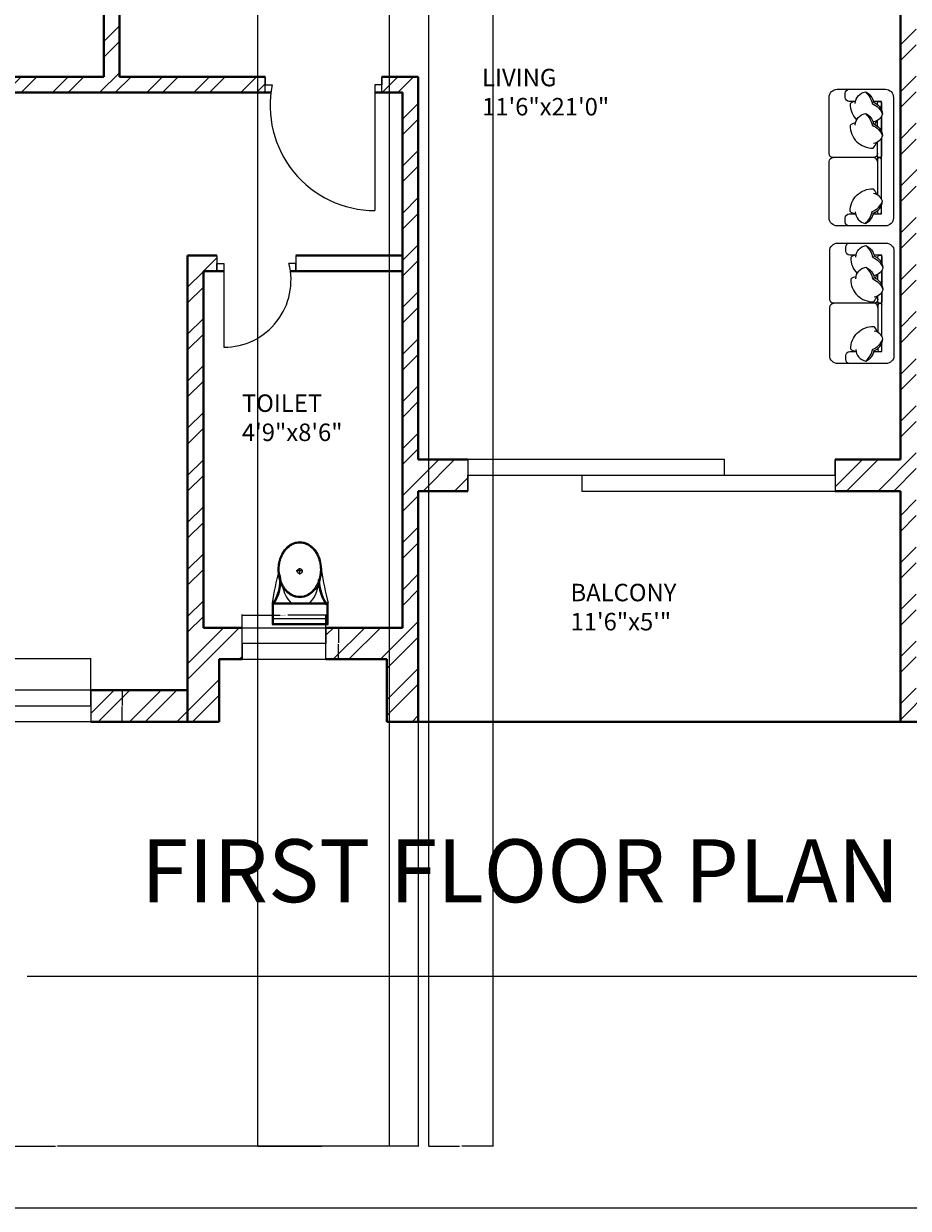
# Model space of a CAD drawing. Units: inches. Extents: x 1601 to 2297, y 1496 to 2631.
# Tile 4 of 57: x 1780 to 2033, y 1496 to 1835. Entities that reach past the tile are written whole.
import ezdxf

# ---------------------------------------------------------------- set-up
doc = ezdxf.new("R2010")
doc.units = ezdxf.units.IN
for name, color, linetype, lineweight in [('A-ANNO-DIMS', 2, 'Continuous', 18), ('A-ANNO-TTLB', 7, 'Continuous', 25), ('A-AREA-IDEN', 7, 'Continuous', 18), ('A-DOOR', 21, 'Continuous', 25), ('A-FLOR-FIXT', 9, 'Continuous', 20), ('A-FURN', 8, 'Continuous', 18), ('A-GLAZ', 161, 'Continuous', 20), ('A-WALL', 7, 'Continuous', 40), ('A-WALL-PATT', 215, 'Continuous', 13)]:
    doc.layers.add(name, color=color, linetype=linetype, lineweight=lineweight)
doc.styles.get("Standard").update_dxf_attribs({"font": 'arial.ttf'})
doc.dimstyles.get("Standard").update_dxf_attribs({"dimtxt": 0.18, "dimasz": 0.18, "dimexe": 0.18, "dimexo": 0.0625, "dimgap": 0.09, "dimtad": 0, "dimtih": 1, "dimtoh": 1, "dimdec": 4, "dimzin": 0, "dimdsep": 46, "dimtxsty": 'Standard', "dimcen": 0.09, "dimadec": 0, "dimazin": 0, "dimtfac": 1, "dimtdec": 4, "dimtofl": 0, "dimtmove": 0, "dimatfit": 3, "dimfxl": 1, "dimtolj": 1, "dimtzin": 0, "dimarcsym": 0})

# ---------------------------------------------------------------- blocks, each defined once
blk = doc.blocks.new('A$C31115884')
for p, q in [((283, 498), (223, 498)), ((258, 466), (258, 523)), ((0, 200), (0, 0)), ((520, 200), (0, 200)), ((10, 190), (10, 10)), ((510, 190), (10, 190)), ((510, 10), (510, 190)), ((520, 0), (520, 200)), ((510, 54), (0, 54)), ((10, 10), (510, 10)), ((0, 0), (520, 0))]:
    blk.add_line(p, q)
blk.add_circle((256, 496), 23.6)
for centre, radius, start, end in [((2778, -205), 2807, 165.4549, 171.7133), ((-295, 403), 365, 324.2091, 9.3499), ((-295, 403), 375, 324.2091, 9.3499), ((806, 403), 365, 170.6501, 215.7909), ((3237, 905), 2807, 188.2867, 194.5451), ((384, 406), 293, 190.2774, 224.1564), ((139, 406), 293, 315.8436, 2.6563), ((806, 403), 375, 179.2036, 215.7909)]:
    blk.add_arc(centre, radius, start, end)
blk.add_ellipse((256, 510), major_axis=(0, -261), ratio=0.772727)
blk.add_open_spline([(256, 259), (263, 259), (270, 260), (288, 262), (299, 265), (320, 273), (330, 278), (350, 291), (360, 299), (378, 316), (386, 326), (402, 347), (409, 358), (421, 383), (427, 395), (436, 422), (440, 436), (445, 465), (447, 480), (448, 509), (448, 524), (445, 553), (443, 568), (436, 596), (432, 610), (422, 636), (416, 649), (402, 672), (395, 683), (379, 703), (370, 712), (351, 728), (341, 735), (321, 746), (310, 751), (289, 757), (278, 759), (256, 761), (245, 761), (223, 757), (212, 754), (191, 746), (181, 741), (161, 728), (151, 720), (133, 703), (125, 693), (110, 672), (103, 660), (90, 636), (85, 623), (76, 596), (72, 582), (67, 553), (66, 538), (64, 509), (65, 494), (68, 465), (70, 450), (77, 422), (81, 408), (91, 382), (97, 370), (111, 346), (118, 335), (135, 316), (144, 307), (162, 291), (172, 284), (193, 273), (203, 269), (225, 262), (236, 260), (250, 259), (253, 259), (256, 259)], degree=3, knots=[0, 0, 0, 0, 0.110105, 0.110105, 0.285049, 0.285049, 0.459994, 0.459994, 0.634938, 0.634938, 0.809882, 0.809882, 0.984827, 0.984827, 1.159771, 1.159771, 1.334715, 1.334715, 1.50966, 1.50966, 1.684604, 1.684604, 1.859549, 1.859549, 2.034493, 2.034493, 2.209437, 2.209437, 2.384382, 2.384382, 2.559326, 2.559326, 2.73427, 2.73427, 2.909215, 2.909215, 3.084159, 3.084159, 3.259103, 3.259103, 3.434048, 3.434048, 3.608992, 3.608992, 3.783936, 3.783936, 3.958881, 3.958881, 4.133825, 4.133825, 4.30877, 4.30877, 4.483714, 4.483714, 4.658658, 4.658658, 4.833603, 4.833603, 5.008547, 5.008547, 5.183491, 5.183491, 5.358436, 5.358436, 5.53338, 5.53338, 5.708324, 5.708324, 5.883269, 5.883269, 6.058213, 6.058213, 6.233158, 6.233158, 6.283185, 6.283185, 6.283185, 6.283185])
blk = doc.blocks.new('WIN-60IN-JAMB9')
for p, q in [((4.5, 60), (0, 60)), ((0, 60), (9, 60)), ((0, 60), (0, 0)), ((4.5, 0), (4.5, 60)), ((9, 60), (9, 0)), ((0, 0), (9, 0)), ((9, 0), (4.5, 0))]:
    blk.add_line(p, q)
blk = doc.blocks.new('WIN-24IN-JAMB9')
for p, q in [((4.5, 24), (0, 24)), ((0, 24), (9, 24)), ((0, 24), (0, 0)), ((4.5, 0), (4.5, 24)), ((9, 24), (9, 0)), ((0, 0), (9, 0)), ((9, 0), (4.5, 0))]:
    blk.add_line(p, q)
blk = doc.blocks.new('*D14')
at = {"layer": 'A-ANNO-DIMS', "color": 0, "lineweight": -2, "transparency": 16777216}
for p, q in [((1739.33, 1644.39), (1739.33, 1653.51)), ((1739.51, 1653.33), (1768.22, 1653.33)), ((1799.15, 1653.33), (1770.45, 1653.33)), ((1799.33, 1644.39), (1799.33, 1653.51))]:
    blk.add_line(p, q, dxfattribs=at)
at = {"layer": 'A-ANNO-DIMS', "color": 0, "transparency": 16777216}
for points in [[(1739.51, 1653.36), (1739.51, 1653.3), (1739.33, 1653.33)], [(1799.15, 1653.36), (1799.15, 1653.3), (1799.33, 1653.33)]]:
    blk.add_solid(points, dxfattribs=at)
at = {"layer": 'Defpoints', "color": 0, "transparency": 16777216}
for p in [(1799.33, 1653.33), (1739.33, 1644.33), (1799.33, 1644.33)]:
    blk.add_point(p, dxfattribs=at)
at = {"layer": 'A-ANNO-DIMS', "color": 0, "transparency": 16777216, "insert": (1769.33, 1653.33), "char_height": 0.18, "attachment_point": 5}
blk.add_mtext('\\A1;WINDOW 60 TYP.', dxfattribs=at)
blk = doc.blocks.new('*D15')
at = {"layer": 'A-ANNO-DIMS', "color": 0, "lineweight": -2, "transparency": 16777216}
for p, q in [((1799.4, 1644.33), (1808.51, 1644.33)), ((1808.33, 1644.15), (1808.33, 1640.01)), ((1808.33, 1635.51), (1808.33, 1639.64)), ((1799.4, 1635.33), (1808.51, 1635.33))]:
    blk.add_line(p, q, dxfattribs=at)
at = {"layer": 'A-ANNO-DIMS', "color": 0, "transparency": 16777216}
for points in [[(1808.3, 1644.15), (1808.36, 1644.15), (1808.33, 1644.33)], [(1808.3, 1635.51), (1808.36, 1635.51), (1808.33, 1635.33)]]:
    blk.add_solid(points, dxfattribs=at)
at = {"layer": 'Defpoints', "color": 0, "transparency": 16777216}
for p in [(1799.33, 1644.33), (1799.33, 1635.33), (1808.33, 1635.33)]:
    blk.add_point(p, dxfattribs=at)
at = {"layer": 'A-ANNO-DIMS', "color": 0, "transparency": 16777216, "insert": (1808.33, 1639.83), "char_height": 0.18, "attachment_point": 5}
blk.add_mtext('\\A1;9 TYP.', dxfattribs=at)
blk = doc.blocks.new('*D26')
at = {"layer": 'A-ANNO-DIMS', "color": 0, "lineweight": -2, "transparency": 16777216}
for p, q in [((1842.62, 1662.27), (1842.62, 1665.98)), ((1842.8, 1665.8), (1853.5, 1665.8)), ((1866.44, 1665.8), (1855.74, 1665.8)), ((1866.62, 1662.27), (1866.62, 1665.98))]:
    blk.add_line(p, q, dxfattribs=at)
at = {"layer": 'A-ANNO-DIMS', "color": 0, "transparency": 16777216}
for points in [[(1842.8, 1665.83), (1842.8, 1665.77), (1842.62, 1665.8)], [(1866.44, 1665.83), (1866.44, 1665.77), (1866.62, 1665.8)]]:
    blk.add_solid(points, dxfattribs=at)
at = {"layer": 'Defpoints', "color": 0, "transparency": 16777216}
for p in [(1842.62, 1665.8), (1842.62, 1662.2), (1866.62, 1662.2)]:
    blk.add_point(p, dxfattribs=at)
at = {"layer": 'A-ANNO-DIMS', "color": 0, "transparency": 16777216, "insert": (1854.62, 1665.8), "char_height": 0.18, "attachment_point": 5}
blk.add_mtext('\\A1;WINDOW 24 TYP.', dxfattribs=at)
blk = doc.blocks.new('*D27')
at = {"layer": 'A-ANNO-DIMS', "color": 0, "lineweight": -2, "transparency": 16777216}
for p, q in [((1866.68, 1662.2), (1870.4, 1662.2)), ((1870.22, 1662.02), (1870.22, 1657.89)), ((1870.22, 1653.38), (1870.22, 1657.52)), ((1866.68, 1653.2), (1870.4, 1653.2))]:
    blk.add_line(p, q, dxfattribs=at)
at = {"layer": 'A-ANNO-DIMS', "color": 0, "transparency": 16777216}
for points in [[(1870.19, 1662.02), (1870.25, 1662.02), (1870.22, 1662.2)], [(1870.19, 1653.38), (1870.25, 1653.38), (1870.22, 1653.2)]]:
    blk.add_solid(points, dxfattribs=at)
at = {"layer": 'Defpoints', "color": 0, "transparency": 16777216}
for p in [(1866.62, 1662.2), (1870.22, 1662.2), (1866.62, 1653.2)]:
    blk.add_point(p, dxfattribs=at)
at = {"layer": 'A-ANNO-DIMS', "color": 0, "transparency": 16777216, "insert": (1870.22, 1657.7), "char_height": 0.18, "attachment_point": 5}
blk.add_mtext('\\A1;9 TYP.', dxfattribs=at)
blk = doc.blocks.new('*D34')
at = {"layer": 'A-ANNO-DIMS', "color": 0, "lineweight": -2, "transparency": 16777216}
for p, q in [((1686.04, 1635.26), (1686.04, 1513.75)), ((1893.04, 1635.26), (1893.04, 1513.75)), ((1686.22, 1513.93), (1789.25, 1513.93)), ((1892.86, 1513.93), (1789.83, 1513.93))]:
    blk.add_line(p, q, dxfattribs=at)
at = {"layer": 'A-ANNO-DIMS', "color": 0, "transparency": 16777216}
for points in [[(1686.22, 1513.96), (1686.22, 1513.9), (1686.04, 1513.93)], [(1892.86, 1513.96), (1892.86, 1513.9), (1893.04, 1513.93)]]:
    blk.add_solid(points, dxfattribs=at)
at = {"layer": 'Defpoints', "color": 0, "transparency": 16777216}
for p in [(1686.04, 1635.33), (1893.04, 1635.33), (1893.04, 1513.93)]:
    blk.add_point(p, dxfattribs=at)
at = {"layer": 'A-ANNO-DIMS', "color": 0, "transparency": 16777216, "insert": (1789.54, 1513.93), "char_height": 0.18, "attachment_point": 5}
blk.add_mtext('\\A1;207', dxfattribs=at)
blk = doc.blocks.new('*D46')
at = {"layer": 'A-ANNO-DIMS', "color": 0, "lineweight": -2, "transparency": 16777216}
for p, q in [((1846.99, 2347.76), (1846.99, 1513.75)), ((1884.68, 2347.76), (1884.68, 1513.75)), ((1847.17, 1513.93), (1865.44, 1513.93)), ((1884.5, 1513.93), (1866.23, 1513.93))]:
    blk.add_line(p, q, dxfattribs=at)
at = {"layer": 'A-ANNO-DIMS', "color": 0, "transparency": 16777216}
for points in [[(1847.17, 1513.96), (1847.17, 1513.9), (1846.99, 1513.93)], [(1884.5, 1513.96), (1884.5, 1513.9), (1884.68, 1513.93)]]:
    blk.add_solid(points, dxfattribs=at)
at = {"layer": 'Defpoints', "color": 0, "transparency": 16777216}
for p in [(1846.99, 2347.83), (1884.68, 2347.83), (1884.68, 1513.93)]:
    blk.add_point(p, dxfattribs=at)
at = {"layer": 'A-ANNO-DIMS', "color": 0, "transparency": 16777216, "insert": (1865.84, 1513.93), "char_height": 0.18, "attachment_point": 5}
blk.add_mtext('\\A1;37.68', dxfattribs=at)
blk = doc.blocks.new('*D50')
at = {"layer": 'A-ANNO-DIMS', "color": 0, "lineweight": -2, "transparency": 16777216}
for p, q in [((1895.99, 2374.33), (1895.99, 1513.75)), ((1914.39, 2374.33), (1914.39, 1513.75)), ((1896.17, 1513.93), (1904.87, 1513.93)), ((1914.21, 1513.93), (1905.5, 1513.93))]:
    blk.add_line(p, q, dxfattribs=at)
at = {"layer": 'A-ANNO-DIMS', "color": 0, "transparency": 16777216}
for points in [[(1896.17, 1513.96), (1896.17, 1513.9), (1895.99, 1513.93)], [(1914.21, 1513.96), (1914.21, 1513.9), (1914.39, 1513.93)]]:
    blk.add_solid(points, dxfattribs=at)
at = {"layer": 'Defpoints', "color": 0, "transparency": 16777216}
for p in [(1895.99, 2374.4), (1914.39, 2374.4), (1914.39, 1513.93)]:
    blk.add_point(p, dxfattribs=at)
at = {"layer": 'A-ANNO-DIMS', "color": 0, "transparency": 16777216, "insert": (1905.19, 1513.93), "char_height": 0.18, "attachment_point": 5}
blk.add_mtext('\\A1;18.4', dxfattribs=at)

msp = doc.modelspace()

# ---------------------------------------------------------------- hatches: boundary and pattern name
at = {"layer": 'A-WALL-PATT'}
h = msp.add_hatch(dxfattribs=at)
h.set_pattern_fill('ANSI32', color=256)
h.paths.add_polyline_path([(1842.0336, 2528.0767), (1842.0336, 2532.3254), (1686.0373, 2532.3254), (1686.0373, 2492.9493), (1695.0373, 2492.9493), (1695.0373, 2523.3254), (1827.0373, 2523.3254), (1827.0373, 2416.8254), (1834.6225, 2416.8254), (1834.6225, 2419.0754), (1834.6225, 2421.3254), (1831.5373, 2421.3254), (1831.5373, 2523.3254), (1842.0336, 2523.3254)])
h.paths.add_polyline_path([(1695.0373, 2432.9493), (1686.0373, 2432.9493), (1686.0373, 2325.989), (1695.0373, 2325.989), (1695.0373, 2347.8254), (1827.0373, 2347.8254), (1827.0373, 2287.8254), (1823.2991, 2287.8254), (1823.2991, 2283.3254), (1847.9422, 2283.3254), (1847.9422, 2285.5754), (1847.9422, 2287.8254), (1831.5373, 2287.8254), (1831.5373, 2347.8254), (1846.9946, 2347.8254), (1846.9946, 2350.0754), (1846.9946, 2352.3254), (1695.0373, 2352.3254)])
h.paths.add_polyline_path([(1807.1169, 1573.5395), (2055.0405, 1573.5395), (2055.0405, 1610.6322), (1807.1169, 1610.6322)], flags=9)
h.paths.add_polyline_path([(1841.1631, 1712.7967), (1870.3957, 1712.7967), (1870.3957, 1731.454), (1841.1631, 1731.454)], flags=9)
h.paths.add_polyline_path([(2144.3862, 1772.185), (2191.0233, 1772.185), (2191.0233, 1790.8423), (2144.3862, 1790.8423)], flags=9)
h.paths.add_polyline_path([(2143.0128, 1827.3312), (2177.9958, 1827.3312), (2177.9958, 1845.9886), (2143.0128, 1845.9886)], flags=9)
h.paths.add_polyline_path([(2041.2439, 1833.5691), (2070.8516, 1833.5691), (2070.8516, 1852.2264), (2041.2439, 1852.2264)], flags=9)
h.paths.add_polyline_path([(2097.2791, 1947.0598), (2134.2061, 1947.0598), (2134.2061, 1965.7171), (2097.2791, 1965.7171)], flags=9)
h.paths.add_polyline_path([(2214.995, 1904.3124), (2214.995, 1942.2899), (2196.3376, 1942.2899), (2196.3376, 1904.3124)], flags=9)
h.paths.add_polyline_path([(2186.6284, 2043.8031), (2219.7935, 2043.8031), (2219.7935, 2062.4605), (2186.6284, 2062.4605)], flags=9)
h.paths.add_polyline_path([(2064.0877, 2031.616), (2097.4949, 2031.616), (2097.4949, 2050.2734), (2064.0877, 2050.2734)], flags=9)
h.paths.add_polyline_path([(1973.1349, 1986.0688), (2008.4009, 1986.0688), (2008.4009, 2004.7261), (1973.1349, 2004.7261)], flags=9)
h.paths.add_polyline_path([(1976.3676, 2106.9635), (2005.7469, 2106.9635), (2005.7469, 2125.6209), (1976.3676, 2125.6209)], flags=9)
h.paths.add_polyline_path([(1991.7852, 2180.4863), (2027.0513, 2180.4863), (2027.0513, 2199.1437), (1991.7852, 2199.1437)], flags=9)
h.paths.add_polyline_path([(2106.1801, 2187.9359), (2152.2101, 2187.9359), (2152.2101, 2206.5932), (2106.1801, 2206.5932)], flags=9)
h.paths.add_polyline_path([(2148.6686, 2262.2542), (2182.318, 2262.2542), (2182.318, 2280.9115), (2148.6686, 2280.9115)], flags=9)
h.paths.add_polyline_path([(2041.6327, 2252.8147), (2071.2405, 2252.8147), (2071.2405, 2271.4721), (2041.6327, 2271.4721)], flags=9)
h.paths.add_polyline_path([(2063.9734, 2375.4265), (2100.9004, 2375.4265), (2100.9004, 2394.0839), (2063.9734, 2394.0839)], flags=9)
h.paths.add_polyline_path([(2216.4955, 2330.9748), (2216.4955, 2370.2654), (2197.8381, 2370.2654), (2197.8381, 2330.9748)], flags=9)
h.paths.add_polyline_path([(2179.1416, 2485.8687), (2212.3067, 2485.8687), (2212.3067, 2504.5261), (2179.1416, 2504.5261)], flags=9)
h.paths.add_polyline_path([(2078.7442, 2471.1516), (2112.1514, 2471.1516), (2112.1514, 2489.809), (2078.7442, 2489.809)], flags=9)
h.paths.add_polyline_path([(1915.9631, 2329.4668), (1952.8902, 2329.4668), (1952.8902, 2348.1241), (1915.9631, 2348.1241)], flags=9)
h.paths.add_polyline_path([(1904.3189, 2499.6709), (1940.4512, 2499.6709), (1940.4512, 2518.3282), (1904.3189, 2518.3282)], flags=9)
h.paths.add_polyline_path([(1892.3665, 2100.4595), (1925.6374, 2100.4595), (1925.6374, 2119.1169), (1892.3665, 2119.1169)], flags=9)
h.paths.add_polyline_path([(1909.2984, 1805.9631), (1946.2254, 1805.9631), (1946.2254, 1824.6205), (1909.2984, 1824.6205)], flags=9)
h.paths.add_polyline_path([(1934.6056, 1658.616), (1970.738, 1658.616), (1970.738, 1677.2733), (1934.6056, 1677.2733)], flags=9)
h.paths.add_polyline_path([(1711.2052, 1789.8902), (1750.0456, 1789.8902), (1750.0456, 1808.5476), (1711.2052, 1808.5476)], flags=9)
h.paths.add_polyline_path([(1742.7874, 1854.6743), (1771.9449, 1854.6743), (1771.9449, 1873.3317), (1742.7874, 1873.3317)], flags=9)
h.paths.add_polyline_path([(1807.3592, 1997.7912), (1850.1116, 1997.7912), (1850.1116, 2016.4486), (1807.3592, 2016.4486)], flags=9)
h.paths.add_polyline_path([(1717.4579, 2237.7844), (1760.2103, 2237.7844), (1760.2103, 2256.4417), (1717.4579, 2256.4417)], flags=9)
h.paths.add_polyline_path([(1780.9285, 2324.0623), (1810.086, 2324.0623), (1810.086, 2342.7197), (1780.9285, 2342.7197)], flags=25)
h.paths.add_polyline_path([(1837.696, 2449.2024), (1866.9286, 2449.2024), (1866.9286, 2467.8598), (1837.696, 2467.8598)], flags=9)
h.paths.add_polyline_path([(1712.7752, 2484.9404), (1751.6156, 2484.9404), (1751.6156, 2503.5977), (1712.7752, 2503.5977)], flags=25)
h = msp.add_hatch(dxfattribs=at)
h.set_pattern_fill('ANSI32', color=256)
h.paths.add_polyline_path([(1973.9371, 2211.3254), (1893.0373, 2211.3254), (1893.0373, 2287.8254), (1884.6167, 2287.8254), (1884.6167, 2285.5754), (1884.6167, 2283.3254), (1888.5373, 2283.3254), (1888.5373, 2145.3254), (1695.0373, 2145.3254), (1695.0373, 2173.8724), (1690.5373, 2173.8724), (1686.0373, 2173.8724), (1686.0373, 2136.3254), (1722.5687, 2136.3254), (1722.5687, 2117.4352), (1731.5687, 2117.4352), (1731.5687, 2136.3254), (1893.0373, 2136.3254), (1893.0373, 2202.3254), (1959.0373, 2202.3254), (1959.0373, 2182.1303), (1968.0373, 2182.1303), (1968.0373, 2202.3254), (1973.9371, 2202.3254)])
h.paths.add_polyline_path([(2094.0373, 2274.6364), (2096.4294, 2274.6364), (2096.4294, 2276.8864), (2096.4294, 2279.1364), (2094.0373, 2279.1364), (2094.0373, 2290.8254), (2094.0373, 2295.3254), (2089.5373, 2295.3254), (2089.5373, 2230.8254), (2035.5373, 2230.8254), (2035.5373, 2299.8254), (2031.0373, 2299.8254), (2031.0373, 2211.3254), (2023.0065, 2211.3254), (2023.0065, 2202.3254), (2031.0373, 2202.3254), (2031.0373, 2140.8254), (1968.0373, 2140.8254), (1968.0373, 2145.9106), (1963.5373, 2145.9106), (1959.0373, 2145.9106), (1959.0373, 2116.839), (1963.5373, 2116.839), (1968.0373, 2116.839), (1968.0373, 2131.8254), (2031.0373, 2131.8254), (2031.0373, 2094.3254), (2031.0373, 2085.3254), (2031.0373, 2056.8254), (1968.0373, 2056.8254), (1968.0373, 2070.4947), (1963.5373, 2070.4947), (1959.0373, 2070.4947), (1959.0373, 2040.3029), (1968.0373, 2040.3029), (1968.0373, 2047.8254), (2031.0373, 2047.8254), (2031.0373, 1983.3254), (2031.0373, 1978.8254), (2021.1979, 1978.8254), (2021.1979, 1974.3254), (2031.0373, 1974.3254), (2031.0373, 1954.3528), (2035.5373, 1954.3528), (2035.5373, 1974.3254), (2035.5373, 1981.8254), (2055.5513, 1981.8254), (2055.5513, 1986.3254), (2035.5373, 1986.3254), (2035.5373, 2047.8254), (2040.0373, 2047.8254), (2040.0373, 2085.3254), (2040.0373, 2094.3254), (2040.0373, 2140.8254), (2035.5373, 2140.8254), (2035.5373, 2226.3254), (2089.5373, 2226.3254), (2094.0373, 2226.3254)])
h.paths.add_polyline_path([(2226.0373, 2230.8254), (2134.5373, 2230.8254), (2134.5373, 2233.5437), (2130.0373, 2233.5437), (2130.0373, 2226.3254), (2134.5373, 2226.3254), (2226.0373, 2226.3254)])
h.paths.add_polyline_path([(1807.1169, 1573.5395), (2055.0405, 1573.5395), (2055.0405, 1610.6322), (1807.1169, 1610.6322)], flags=9)
h.paths.add_polyline_path([(1841.1631, 1712.7967), (1870.3957, 1712.7967), (1870.3957, 1731.454), (1841.1631, 1731.454)], flags=9)
h.paths.add_polyline_path([(2144.3862, 1772.185), (2191.0233, 1772.185), (2191.0233, 1790.8423), (2144.3862, 1790.8423)], flags=9)
h.paths.add_polyline_path([(2143.0128, 1827.3312), (2177.9958, 1827.3312), (2177.9958, 1845.9886), (2143.0128, 1845.9886)], flags=9)
h.paths.add_polyline_path([(2041.2439, 1833.5691), (2070.8516, 1833.5691), (2070.8516, 1852.2264), (2041.2439, 1852.2264)], flags=9)
h.paths.add_polyline_path([(2097.2791, 1947.0598), (2134.2061, 1947.0598), (2134.2061, 1965.7171), (2097.2791, 1965.7171)], flags=9)
h.paths.add_polyline_path([(2214.995, 1904.3124), (2214.995, 1942.2899), (2196.3376, 1942.2899), (2196.3376, 1904.3124)], flags=9)
h.paths.add_polyline_path([(2186.6284, 2043.8031), (2219.7935, 2043.8031), (2219.7935, 2062.4605), (2186.6284, 2062.4605)], flags=9)
h.paths.add_polyline_path([(2064.0877, 2031.616), (2097.4949, 2031.616), (2097.4949, 2050.2734), (2064.0877, 2050.2734)], flags=9)
h.paths.add_polyline_path([(1973.1349, 1986.0688), (2008.4009, 1986.0688), (2008.4009, 2004.7261), (1973.1349, 2004.7261)], flags=25)
h.paths.add_polyline_path([(1976.3676, 2106.9635), (2005.7469, 2106.9635), (2005.7469, 2125.6209), (1976.3676, 2125.6209)], flags=25)
h.paths.add_polyline_path([(1991.7852, 2180.4863), (2027.0513, 2180.4863), (2027.0513, 2199.1437), (1991.7852, 2199.1437)], flags=25)
h.paths.add_polyline_path([(2106.1801, 2187.9359), (2152.2101, 2187.9359), (2152.2101, 2206.5932), (2106.1801, 2206.5932)], flags=9)
h.paths.add_polyline_path([(2148.6686, 2262.2542), (2182.318, 2262.2542), (2182.318, 2280.9115), (2148.6686, 2280.9115)], flags=9)
h.paths.add_polyline_path([(2041.6327, 2252.8147), (2071.2405, 2252.8147), (2071.2405, 2271.4721), (2041.6327, 2271.4721)], flags=25)
h.paths.add_polyline_path([(2063.9734, 2375.4265), (2100.9004, 2375.4265), (2100.9004, 2394.0839), (2063.9734, 2394.0839)], flags=9)
h.paths.add_polyline_path([(2216.4955, 2330.9748), (2216.4955, 2370.2654), (2197.8381, 2370.2654), (2197.8381, 2330.9748)], flags=9)
h.paths.add_polyline_path([(2179.1416, 2485.8687), (2212.3067, 2485.8687), (2212.3067, 2504.5261), (2179.1416, 2504.5261)], flags=9)
h.paths.add_polyline_path([(2078.7442, 2471.1516), (2112.1514, 2471.1516), (2112.1514, 2489.809), (2078.7442, 2489.809)], flags=9)
h.paths.add_polyline_path([(1915.9631, 2329.4668), (1952.8902, 2329.4668), (1952.8902, 2348.1241), (1915.9631, 2348.1241)], flags=9)
h.paths.add_polyline_path([(1904.3189, 2499.6709), (1940.4512, 2499.6709), (1940.4512, 2518.3282), (1904.3189, 2518.3282)], flags=9)
h.paths.add_polyline_path([(1892.3665, 2100.4595), (1925.6374, 2100.4595), (1925.6374, 2119.1169), (1892.3665, 2119.1169)], flags=9)
h.paths.add_polyline_path([(1909.2984, 1805.9631), (1946.2254, 1805.9631), (1946.2254, 1824.6205), (1909.2984, 1824.6205)], flags=9)
h.paths.add_polyline_path([(1934.6056, 1658.616), (1970.738, 1658.616), (1970.738, 1677.2733), (1934.6056, 1677.2733)], flags=9)
h.paths.add_polyline_path([(1711.2052, 1789.8902), (1750.0456, 1789.8902), (1750.0456, 1808.5476), (1711.2052, 1808.5476)], flags=9)
h.paths.add_polyline_path([(1742.7874, 1854.6743), (1771.9449, 1854.6743), (1771.9449, 1873.3317), (1742.7874, 1873.3317)], flags=9)
h.paths.add_polyline_path([(1807.3592, 1997.7912), (1850.1116, 1997.7912), (1850.1116, 2016.4486), (1807.3592, 2016.4486)], flags=9)
h.paths.add_polyline_path([(1717.4579, 2237.7844), (1760.2103, 2237.7844), (1760.2103, 2256.4417), (1717.4579, 2256.4417)], flags=25)
h.paths.add_polyline_path([(1780.9285, 2324.0623), (1810.086, 2324.0623), (1810.086, 2342.7197), (1780.9285, 2342.7197)], flags=9)
h.paths.add_polyline_path([(1837.696, 2449.2024), (1866.9286, 2449.2024), (1866.9286, 2467.8598), (1837.696, 2467.8598)], flags=9)
h.paths.add_polyline_path([(1712.7752, 2484.9404), (1751.6156, 2484.9404), (1751.6156, 2503.5977), (1712.7752, 2503.5977)], flags=9)
h = msp.add_hatch(dxfattribs=at)
h.set_pattern_fill('ANSI32', color=256)
h.paths.add_polyline_path([(2230.5373, 1861.8254), (2182.5373, 1861.8254), (2182.5373, 1885.3637), (2178.0373, 1885.3637), (2178.0373, 1861.8254), (2166.0373, 1861.8254), (2134.5373, 1861.8254), (2130.0373, 1861.8254), (2130.0373, 1841.4682), (2126.8833, 1841.4682), (2126.8833, 1836.9682), (2130.0373, 1836.9682), (2130.0373, 1822.7302), (2134.5373, 1822.7302), (2134.5373, 1857.3254), (2166.0373, 1857.3254), (2226.0373, 1857.3254), (2226.0373, 1846.1155), (2230.5373, 1846.1155)])
h.paths.add_polyline_path([(2226.0373, 1797.3254), (2134.5373, 1797.3254), (2134.5373, 1800.6636), (2132.2873, 1800.6636), (2130.0373, 1800.6636), (2130.0373, 1797.3254), (2130.0373, 1792.8254), (2167.7264, 1792.8254), (2226.0373, 1792.8254)])
h.paths.add_polyline_path([(2230.5373, 1822.1155), (2226.0373, 1822.1155), (2226.0373, 1760.8563), (2230.5373, 1760.8563)])
h.paths.add_polyline_path([(2230.5373, 1700.8563), (2226.0373, 1700.8563), (2226.0373, 1644.3254), (2140.2517, 1644.3254), (2140.2517, 1635.3254), (2230.5373, 1635.3254)])
h.paths.add_polyline_path([(2080.2517, 1639.8254), (2080.2517, 1644.3254), (2035.5373, 1644.3254), (2035.5373, 1792.8254), (2094.0373, 1792.8254), (2094.0373, 1797.3254), (2094.0373, 1836.9682), (2097.1057, 1836.9682), (2097.1057, 1839.2182), (2097.1057, 1841.4682), (2094.0373, 1841.4682), (2094.0373, 1862.2276), (2089.5373, 1862.2276), (2089.5373, 1797.3254), (2035.5373, 1797.3254), (2035.5373, 1857.3254), (2035.5373, 1885.0916), (2031.0373, 1885.0916), (2031.0373, 1710.3254), (2012.329, 1710.3254), (2012.329, 1701.3254), (2031.0373, 1701.3254), (2031.0373, 1644.3254), (2031.0373, 1635.3254), (2080.2517, 1635.3254)])
h.paths.add_polyline_path([(1836.0373, 1653.2033), (1842.6171, 1653.2033), (1842.6171, 1657.7033), (1842.6171, 1662.2033), (1831.5373, 1662.2033), (1831.5373, 1764.2033), (1835.3881, 1764.2033), (1835.3881, 1766.4533), (1835.3881, 1768.7033), (1831.5373, 1768.7033), (1827.0373, 1768.7033), (1827.0373, 1662.2033), (1827.0373, 1635.3254), (1836.0373, 1635.3254)])
h.paths.add_polyline_path([(1893.0373, 1701.3254), (1907.193, 1701.3254), (1907.193, 1705.8254), (1907.193, 1710.3254), (1893.0373, 1710.3254), (1893.0373, 1819.8254), (1882.6444, 1819.8254), (1882.6444, 1817.5754), (1882.6444, 1815.3254), (1888.5373, 1815.3254), (1888.5373, 1662.2033), (1884.0373, 1662.2033), (1866.6171, 1662.2033), (1866.6171, 1653.2033), (1882.391, 1653.2033), (1884.0373, 1653.2033), (1884.0373, 1635.3254), (1893.0373, 1635.3254)])
h.paths.add_polyline_path([(1739.3335, 1639.8254), (1739.3335, 1644.3254), (1695.0373, 1644.3254), (1695.0373, 1702.0135), (1690.5373, 1702.0135), (1686.0373, 1702.0135), (1686.0373, 1635.3254), (1739.3335, 1635.3254)])
h.paths.add_polyline_path([(1827.0373, 1644.3254), (1799.3335, 1644.3254), (1799.3335, 1635.3254), (1827.0373, 1635.3254)])
h.paths.add_polyline_path([(1695.0373, 1815.3254), (1849.2759, 1815.3254), (1849.2759, 1819.8254), (1807.5373, 1819.8254), (1807.5373, 1879.8254), (1851.1533, 1879.8254), (1851.1533, 1882.0754), (1851.1533, 1884.3254), (1799.3405, 1884.3254), (1799.3405, 1882.0754), (1799.3405, 1879.8254), (1803.0373, 1879.8254), (1803.0373, 1819.8254), (1695.0373, 1819.8254), (1695.0373, 1835.0458), (1690.5373, 1835.0458), (1686.0373, 1835.0458), (1686.0373, 1766.1753), (1695.0373, 1766.1753)])
h.paths.add_polyline_path([(1775.8157, 1884.3254), (1695.0373, 1884.3254), (1695.0373, 1912.9526), (1690.5373, 1912.9526), (1686.0373, 1912.9526), (1686.0373, 1859.0458), (1695.0373, 1859.0458), (1695.0373, 1879.8254), (1775.8157, 1879.8254)])
h.paths.add_polyline_path([(1893.0373, 2031.3254), (1731.5687, 2031.3254), (1731.5687, 2057.4352), (1722.5687, 2057.4352), (1722.5687, 2031.3254), (1686.0373, 2031.3254), (1686.0373, 1972.9526), (1695.0373, 1972.9526), (1695.0373, 2022.3254), (1888.5373, 2022.3254), (1888.5373, 1884.3254), (1883.4996, 1884.3254), (1883.4996, 1879.8254), (1893.0373, 1879.8254), (1893.0373, 1974.3254), (1976.6199, 1974.3254), (1976.6199, 1978.8254), (1968.0373, 1978.8254), (1968.0373, 1983.3254), (1968.0373, 2008.4756), (1963.5373, 2008.4756), (1959.0373, 2008.4756), (1959.0373, 1983.3254), (1893.0373, 1983.3254)])
h.paths.add_polyline_path([(2230.5373, 2140.4745), (2226.0373, 2140.4745), (2226.0373, 2094.3254), (2040.0373, 2094.3254), (2040.0373, 2085.3254), (2178.0373, 2085.3254), (2178.0373, 2065.6965), (2182.5373, 2065.6965), (2182.5373, 2085.3254), (2226.0373, 2085.3254), (2226.0373, 1986.3254), (2211.2679, 1986.3254), (2211.2679, 1981.8254), (2230.5373, 1981.8254)])
h.paths.add_polyline_path([(2187.6292, 1986.3254), (2182.5373, 1986.3254), (2182.5373, 2029.6965), (2178.0373, 2029.6965), (2178.0373, 1986.3254), (2099.05, 1986.3254), (2099.05, 1981.8254), (2178.0373, 1981.8254), (2178.0373, 1969.3637), (2182.5373, 1969.3637), (2182.5373, 1981.8254), (2187.6292, 1981.8254), (2187.6292, 1984.0754)])
h.paths.add_polyline_path([(1807.1169, 1573.5395), (2055.0405, 1573.5395), (2055.0405, 1610.6322), (1807.1169, 1610.6322)], flags=9)
h.paths.add_polyline_path([(1841.1631, 1712.7967), (1870.3957, 1712.7967), (1870.3957, 1731.454), (1841.1631, 1731.454)], flags=9)
h.paths.add_polyline_path([(2144.3862, 1772.185), (2191.0233, 1772.185), (2191.0233, 1790.8423), (2144.3862, 1790.8423)], flags=9)
h.paths.add_polyline_path([(2143.0128, 1827.3312), (2177.9958, 1827.3312), (2177.9958, 1845.9886), (2143.0128, 1845.9886)], flags=25)
h.paths.add_polyline_path([(2041.2439, 1833.5691), (2070.8516, 1833.5691), (2070.8516, 1852.2264), (2041.2439, 1852.2264)], flags=25)
h.paths.add_polyline_path([(2097.2791, 1947.0598), (2134.2061, 1947.0598), (2134.2061, 1965.7171), (2097.2791, 1965.7171)], flags=9)
h.paths.add_polyline_path([(2214.995, 1904.3124), (2214.995, 1942.2899), (2196.3376, 1942.2899), (2196.3376, 1904.3124)], flags=9)
h.paths.add_polyline_path([(2186.6284, 2043.8031), (2219.7935, 2043.8031), (2219.7935, 2062.4605), (2186.6284, 2062.4605)], flags=25)
h.paths.add_polyline_path([(2064.0877, 2031.616), (2097.4949, 2031.616), (2097.4949, 2050.2734), (2064.0877, 2050.2734)], flags=25)
h.paths.add_polyline_path([(1973.1349, 1986.0688), (2008.4009, 1986.0688), (2008.4009, 2004.7261), (1973.1349, 2004.7261)], flags=9)
h.paths.add_polyline_path([(1976.3676, 2106.9635), (2005.7469, 2106.9635), (2005.7469, 2125.6209), (1976.3676, 2125.6209)], flags=9)
h.paths.add_polyline_path([(1991.7852, 2180.4863), (2027.0513, 2180.4863), (2027.0513, 2199.1437), (1991.7852, 2199.1437)], flags=9)
h.paths.add_polyline_path([(2106.1801, 2187.9359), (2152.2101, 2187.9359), (2152.2101, 2206.5932), (2106.1801, 2206.5932)], flags=9)
h.paths.add_polyline_path([(2148.6686, 2262.2542), (2182.318, 2262.2542), (2182.318, 2280.9115), (2148.6686, 2280.9115)], flags=9)
h.paths.add_polyline_path([(2041.6327, 2252.8147), (2071.2405, 2252.8147), (2071.2405, 2271.4721), (2041.6327, 2271.4721)], flags=9)
h.paths.add_polyline_path([(2063.9734, 2375.4265), (2100.9004, 2375.4265), (2100.9004, 2394.0839), (2063.9734, 2394.0839)], flags=9)
h.paths.add_polyline_path([(2216.4955, 2330.9748), (2216.4955, 2370.2654), (2197.8381, 2370.2654), (2197.8381, 2330.9748)], flags=9)
h.paths.add_polyline_path([(2179.1416, 2485.8687), (2212.3067, 2485.8687), (2212.3067, 2504.5261), (2179.1416, 2504.5261)], flags=9)
h.paths.add_polyline_path([(2078.7442, 2471.1516), (2112.1514, 2471.1516), (2112.1514, 2489.809), (2078.7442, 2489.809)], flags=9)
h.paths.add_polyline_path([(1915.9631, 2329.4668), (1952.8902, 2329.4668), (1952.8902, 2348.1241), (1915.9631, 2348.1241)], flags=9)
h.paths.add_polyline_path([(1904.3189, 2499.6709), (1940.4512, 2499.6709), (1940.4512, 2518.3282), (1904.3189, 2518.3282)], flags=9)
h.paths.add_polyline_path([(1892.3665, 2100.4595), (1925.6374, 2100.4595), (1925.6374, 2119.1169), (1892.3665, 2119.1169)], flags=9)
h.paths.add_polyline_path([(1909.2984, 1805.9631), (1946.2254, 1805.9631), (1946.2254, 1824.6205), (1909.2984, 1824.6205)], flags=9)
h.paths.add_polyline_path([(1934.6056, 1658.616), (1970.738, 1658.616), (1970.738, 1677.2733), (1934.6056, 1677.2733)], flags=9)
h.paths.add_polyline_path([(1711.2052, 1789.8902), (1750.0456, 1789.8902), (1750.0456, 1808.5476), (1711.2052, 1808.5476)], flags=25)
h.paths.add_polyline_path([(1742.7874, 1854.6743), (1771.9449, 1854.6743), (1771.9449, 1873.3317), (1742.7874, 1873.3317)], flags=25)
h.paths.add_polyline_path([(1807.3592, 1997.7912), (1850.1116, 1997.7912), (1850.1116, 2016.4486), (1807.3592, 2016.4486)], flags=25)
h.paths.add_polyline_path([(1717.4579, 2237.7844), (1760.2103, 2237.7844), (1760.2103, 2256.4417), (1717.4579, 2256.4417)], flags=9)
h.paths.add_polyline_path([(1780.9285, 2324.0623), (1810.086, 2324.0623), (1810.086, 2342.7197), (1780.9285, 2342.7197)], flags=9)
h.paths.add_polyline_path([(1837.696, 2449.2024), (1866.9286, 2449.2024), (1866.9286, 2467.8598), (1837.696, 2467.8598)], flags=9)
h.paths.add_polyline_path([(1712.7752, 2484.9404), (1751.6156, 2484.9404), (1751.6156, 2503.5977), (1712.7752, 2503.5977)], flags=9)

# ---------------------------------------------------------------- linework, layer by layer
at = {"layer": 'A-ANNO-TTLB'}
msp.add_line((1781.0743, 1562.4779), (2069.7201, 1562.4779), dxfattribs=at)
msp.add_lwpolyline([(1600.5933, 2631.1477), (2297.129, 2631.1477), (2297.129, 1496.1026), (1600.5933, 1496.1026)], close=True, dxfattribs=at)
at = {"layer": 'A-DOOR'}
for p, q in [((1849.2759, 1815.3254), (1849.2759, 1819.8254)), ((1849.2759, 1819.8254), (1849.2759, 1817.5754)), ((1849.2759, 1817.5754), (1851.2759, 1817.5754)), ((1882.6444, 1817.5754), (1880.6444, 1817.5754)), ((1880.6444, 1817.5754), (1880.6444, 1781.5754)), ((1882.6444, 1815.3254), (1882.6444, 1819.8254)), ((1882.6444, 1819.8254), (1882.6444, 1817.5754)), ((1835.3881, 1768.7033), (1835.3881, 1764.2033)), ((1835.3881, 1764.2033), (1835.3881, 1766.4533)), ((1835.3881, 1766.4533), (1837.3881, 1766.4533)), ((1837.3881, 1766.4533), (1837.3881, 1742.4533)), ((1858.0379, 1766.4533), (1856.0379, 1766.4533)), ((1858.0379, 1768.7033), (1858.0379, 1764.2033)), ((1858.0379, 1764.2033), (1858.0379, 1766.4533)), ((1907.193, 1710.3254), (1907.193, 1701.3254)), ((1980.6638, 1710.3254), (1907.193, 1710.3254)), ((1980.6638, 1705.8254), (1980.6638, 1710.3254)), ((2012.329, 1705.8254), (2012.329, 1710.3254)), ((2012.329, 1710.3254), (2012.329, 1701.3254)), ((1907.193, 1701.3254), (1907.193, 1705.8254)), ((1907.193, 1705.8254), (2012.329, 1705.8254)), ((1939.8536, 1705.8254), (1939.8536, 1701.3254)), ((1939.8536, 1701.3254), (2012.329, 1701.3254))]:
    msp.add_line(p, q, dxfattribs=at)
for centre, radius, start, end in [((1880.6444, 1811.5547), 29.9793, 168.414643, 270), ((1837.3881, 1761.6994), 19.2461, 270, 14.300282)]:
    msp.add_arc(centre, radius, start, end, dxfattribs=at)
at = {"layer": 'A-FURN', "ltscale": 0.03}
for points in [[(2010.6325, 1795.5746, -0.41421356), (2011.7825, 1796.7245, -0.41421356), (2010.6325, 1797.8745), (2010.6325, 1813.9739, -0.41421356), (2012.9324, 1816.2738), (2026.7319, 1816.2738, -0.41421356), (2029.0318, 1813.9739), (2029.0318, 1779.4752, -0.41421356), (2026.7319, 1777.1752), (2012.9324, 1777.1752, -0.41421356), (2010.6325, 1779.4752), (2010.6325, 1795.5746, -0.41421356), (2011.7825, 1796.7245, -0.41421356), (2010.6325, 1797.8745)], [(2010.787, 1753.888, -0.41421356), (2011.937, 1755.038, -0.41421356), (2010.787, 1756.1879), (2010.787, 1769.9874, -0.41421356), (2013.0869, 1772.2873), (2026.8864, 1772.2873, -0.41421356), (2029.1863, 1769.9874), (2029.1863, 1740.0885, -0.41421356), (2026.8864, 1737.7886), (2013.0869, 1737.7886, -0.41421356), (2010.787, 1740.0885), (2010.787, 1753.888, -0.41421356), (2011.937, 1755.038, -0.41421356), (2010.787, 1756.1879)]]:
    msp.add_lwpolyline(points, format="xyb", dxfattribs=at)
at = {"layer": 'A-FURN'}
for points in [[(2018.164, 1812.8239), (2016.3823, 1812.8239, -0.41421356), (2015.2323, 1813.9739), (2015.2323, 1815.1239, -0.41421356), (2016.3823, 1816.2738)], [(2018.0944, 1812.2468, -0.35677236), (2020.993, 1815.5419, -0.24954205), (2023.3817, 1812.5563, 9.61688035)], [(2020.993, 1815.5419, -0.14772988), (2022.9693, 1812.1809, -0.21334276), (2025.8679, 1809.2154, -0.17866181)], [(2018.1645, 1812.8264, 0.16554063), (2016.6451, 1812.115, 0.20023115), (2018.4956, 1807.5501, 0.12152332)], [(2023.1268, 1812.6453, -0.30666349), (2025.8679, 1809.2154, -0.30632997), (2023.3646, 1806.9747, 0.87284716)], [(2025.582, 1810.4047), (2025.582, 1812.8239), (2023.322, 1812.8239, -0.41421356)], [(2024.432, 1811.9464), (2024.432, 1812.364, -0.41421356), (2024.892, 1812.8239), (2025.122, 1812.8239, -0.41421356), (2025.582, 1812.364)], [(2025.582, 1812.364), (2025.582, 1810.4047, -0.41421356)], [(2018.1645, 1806.6317, 0.16554063), (2016.6451, 1805.9203, 0.42598917), (2023.2328, 1799.4619, 0.12152332), (2024.1408, 1800.995, -7.11546429)], [(2018.0944, 1806.0521, -0.35677236), (2020.993, 1809.3472, -0.24954205), (2023.3817, 1806.3615, 9.61688035)], [(2020.993, 1809.3472, -0.14772988), (2022.9693, 1805.9862, -0.21334276), (2025.8679, 1803.0206, -0.17866181)], [(2023.6913, 1806.2256, 0.07186538), (2024.1408, 1807.1898, -7.11546429)], [(2024.432, 1805.7516), (2024.432, 1807.3337, -0.41421356)], [(2025.582, 1808.4916), (2025.582, 1804.21, -0.41421356)], [(2023.1268, 1806.4505, -0.30666349), (2025.8679, 1803.0206, -0.30632997), (2023.3646, 1800.7799, 0.87284716)], [(2025.582, 1802.2969), (2025.582, 1797.1845, -0.41421356), (2025.122, 1796.7245), (2024.892, 1796.7245, -0.41421356), (2024.432, 1797.1845), (2024.432, 1801.1389, -0.41421356)], [(2024.432, 1797.8745, -0.41421356), (2023.282, 1796.7245), (2011.7825, 1796.7245, -0.41421356)], [(2024.432, 1795.5746, 0.41421356), (2023.282, 1796.7245), (2011.7825, 1796.7245, 0.41421356)], [(2024.432, 1797.8745, -0.41421356), (2023.282, 1796.7245)], [(2024.432, 1795.5746, 0.41421356), (2023.282, 1796.7245)], [(2025.582, 1784.9574), (2025.582, 1796.2645, 0.41421356), (2025.122, 1796.7245), (2024.892, 1796.7245, 0.41421356), (2024.432, 1796.2645), (2024.432, 1786.1154, 0.41421356)], [(2018.1645, 1780.6226, -0.16554063), (2016.6451, 1781.334, -0.42598917), (2023.2328, 1787.7924, -0.12152332), (2024.1408, 1786.2593, 7.11546429)], [(2023.1268, 1780.8038, 0.30666349), (2025.8679, 1784.2337, 0.30632997), (2023.3646, 1786.4744, -0.87284716)], [(2020.993, 1777.9071, 0.14772988), (2022.9693, 1781.2681, 0.21334276), (2025.8679, 1784.2337, 0.17866181)], [(2025.582, 1781.0851), (2025.582, 1783.0443, 0.41421356)], [(2016.3823, 1777.1752, -0.41421356), (2015.2323, 1778.3252), (2015.2323, 1779.4752, -0.41421356), (2016.3823, 1780.6251), (2018.164, 1780.6251)], [(2018.0944, 1781.2022, 0.35677236), (2020.993, 1777.9071, 0.24954205), (2023.3817, 1780.8928, -9.61688035)], [(2024.432, 1781.5027), (2024.432, 1781.0851, 0.41421356), (2024.892, 1780.6251), (2025.122, 1780.6251, 0.41421356), (2025.582, 1781.0851)], [(2018.3185, 1768.8375), (2016.5368, 1768.8375, -0.41421356), (2015.3868, 1769.9874), (2015.3868, 1771.1374, -0.41421356), (2016.5368, 1772.2873)], [(2018.2489, 1768.2604, -0.35677236), (2021.1475, 1771.5555, -0.24954205), (2023.5362, 1768.5698, 9.61688035)], [(2021.1475, 1771.5555, -0.14772988), (2023.1238, 1768.1945, -0.21334276), (2026.0224, 1765.2289, -0.17866181)], [(2018.319, 1768.84, 0.16554063), (2016.7996, 1768.1286, 0.20023115), (2018.6501, 1763.5637, 0.12152332)], [(2023.2813, 1768.6588, -0.30666349), (2026.0224, 1765.2289, -0.30632997), (2023.5191, 1762.9882, 0.87284716)], [(2025.7364, 1766.4183), (2025.7364, 1768.8375), (2023.4765, 1768.8375, -0.41421356)], [(2024.5865, 1767.9599), (2024.5865, 1768.3775, -0.41421356), (2025.0465, 1768.8375), (2025.2765, 1768.8375, -0.41421356), (2025.7364, 1768.3775)], [(2025.7364, 1768.3775), (2025.7364, 1766.4183, -0.41421356)], [(2018.319, 1762.6452, 0.16554063), (2016.7996, 1761.9338, 0.42598917), (2023.3873, 1755.4754, 0.12152332), (2024.2953, 1757.0085, -7.11546429)], [(2018.2489, 1762.0656, -0.35677236), (2021.1475, 1765.3607, -0.24954205), (2023.5362, 1762.375, 9.61688035)], [(2021.1475, 1765.3607, -0.14772988), (2023.1238, 1761.9997, -0.21334276), (2026.0224, 1759.0341, -0.17866181)], [(2023.8457, 1762.2392, 0.07186538), (2024.2953, 1763.2033, -7.11546429)], [(2024.5865, 1761.7651), (2024.5865, 1763.3472, -0.41421356)], [(2025.7364, 1764.5052), (2025.7364, 1760.2235, -0.41421356)], [(2023.2813, 1762.464, -0.30666349), (2026.0224, 1759.0341, -0.30632997), (2023.5191, 1756.7934, 0.87284716)], [(2024.5865, 1756.1879, -0.41421356), (2023.4365, 1755.038), (2011.937, 1755.038, -0.41421356)], [(2024.5865, 1756.1879, -0.41421356), (2023.4365, 1755.038)], [(2025.7364, 1758.3104), (2025.7364, 1755.4979, -0.41421356), (2025.2765, 1755.038), (2025.0465, 1755.038, -0.41421356), (2024.5865, 1755.4979), (2024.5865, 1757.1524, -0.41421356)], [(2024.5865, 1753.888, 0.41421356), (2023.4365, 1755.038), (2011.937, 1755.038, 0.41421356)], [(2024.5865, 1753.888, 0.41421356), (2023.4365, 1755.038)], [(2025.7364, 1745.5708), (2025.7364, 1754.578, 0.41421356), (2025.2765, 1755.038), (2025.0465, 1755.038, 0.41421356), (2024.5865, 1754.578), (2024.5865, 1746.7287, 0.41421356)], [(2018.319, 1741.236, -0.16554063), (2016.7996, 1741.9474, -0.42598917), (2023.3873, 1748.4058, -0.12152332), (2024.2953, 1746.8727, 7.11546429)], [(2023.2813, 1741.4171, 0.30666349), (2026.0224, 1744.8471, 0.30632997), (2023.5191, 1747.0877, -0.87284716)], [(2021.1475, 1738.5205, 0.14772988), (2023.1238, 1741.8815, 0.21334276), (2026.0224, 1744.8471, 0.17866181)], [(2025.7364, 1741.6985), (2025.7364, 1743.6577, 0.41421356)], [(2016.5368, 1737.7886, -0.41421356), (2015.3868, 1738.9386), (2015.3868, 1740.0885, -0.41421356), (2016.5368, 1741.2385), (2018.3185, 1741.2385)], [(2018.2489, 1741.8156, 0.35677236), (2021.1475, 1738.5205, 0.24954205), (2023.5362, 1741.5061, -9.61688035)], [(2024.5865, 1742.116), (2024.5865, 1741.6985, 0.41421356), (2025.0465, 1741.2385), (2025.2765, 1741.2385, 0.41421356), (2025.7364, 1741.6985)]]:
    msp.add_lwpolyline(points, format="xyb", dxfattribs=at)
for points in [[(2025.582, 1804.21), (2025.582, 1808.4916)], [(2025.582, 1784.9574), (2025.582, 1802.2969)], [(2023.322, 1780.6251), (2025.582, 1780.6251), (2025.582, 1783.0443)], [(2025.7364, 1760.2235), (2025.7364, 1764.5052)], [(2025.7364, 1745.5708), (2025.7364, 1758.3104)], [(2023.4765, 1741.2385), (2025.7364, 1741.2385), (2025.7364, 1743.6577)]]:
    msp.add_lwpolyline(points, dxfattribs=at)
for points in [[(2025.582, 1796.2645), (2025.582, 1797.1845, -0.41421356), (2025.122, 1796.7245), (2024.892, 1796.7245, -0.41421356), (2024.432, 1797.1845), (2024.432, 1796.2645, -0.41421356), (2024.892, 1796.7245), (2025.122, 1796.7245, -0.41421356)], [(2025.7364, 1754.578), (2025.7364, 1755.4979, -0.41421356), (2025.2765, 1755.038), (2025.0465, 1755.038, -0.41421356), (2024.5865, 1755.4979), (2024.5865, 1754.578, -0.41421356), (2025.0465, 1755.038), (2025.2765, 1755.038, -0.41421356)]]:
    msp.add_lwpolyline(points, format="xyb", close=True, dxfattribs=at)
at = {"layer": 'A-WALL'}
for p, q in [((2031.0373, 1710.3254), (2031.0373, 1885.0916)), ((1803.0373, 1879.8254), (1803.0373, 1819.8254)), ((1807.5373, 1819.8254), (1807.5373, 1879.8254)), ((1695.0373, 1819.8254), (1803.0373, 1819.8254)), ((1807.5373, 1819.8254), (1849.2759, 1819.8254)), ((1882.6444, 1819.8254), (1893.0373, 1819.8254)), ((1893.0373, 1819.8254), (1893.0373, 1710.3254)), ((1695.0373, 1815.3254), (1850.9031, 1815.3254)), ((1880.6444, 1815.3254), (1888.5373, 1815.3254)), ((1888.5373, 1815.3254), (1888.5373, 1662.2033)), ((1831.5373, 1768.7033), (1827.0373, 1768.7033)), ((1827.0373, 1768.7033), (1827.0373, 1662.2033)), ((1835.3881, 1768.7033), (1831.5373, 1768.7033)), ((1888.5373, 1768.7033), (1858.0379, 1768.7033)), ((1831.5373, 1662.2033), (1831.5373, 1764.2033)), ((1831.5373, 1764.2033), (1837.3881, 1764.2033)), ((1856.4706, 1764.2033), (1888.5373, 1764.2033)), ((1888.5373, 1746.3254), (1888.5373, 1750.8254)), ((1907.193, 1710.3254), (1893.0373, 1710.3254)), ((2031.0373, 1710.3254), (2012.329, 1710.3254)), ((1893.0373, 1635.3254), (1893.0373, 1701.3254)), ((1893.0373, 1701.3254), (1907.193, 1701.3254)), ((1893.0373, 1701.3254), (1893.0373, 1644.3254)), ((2012.329, 1701.3254), (2031.0373, 1701.3254)), ((2031.0373, 1644.3254), (2031.0373, 1701.3254)), ((1827.0373, 1662.2033), (1827.0373, 1635.3254)), ((1831.5373, 1662.2033), (1842.6171, 1662.2033)), ((1831.5373, 1662.2033), (1836.0373, 1662.2033)), ((1866.6171, 1662.2033), (1888.5373, 1662.2033)), ((1888.5373, 1662.2033), (1884.0373, 1662.2033)), ((1836.0373, 1653.2033), (1836.0373, 1635.3254)), ((1836.0373, 1653.2033), (1842.6171, 1653.2033)), ((1866.6171, 1653.2033), (1882.391, 1653.2033)), ((1882.391, 1653.2033), (1884.0373, 1653.2033)), ((1884.0373, 1653.2033), (1884.0373, 1635.3254)), ((1799.3335, 1644.3254), (1827.0373, 1644.3254)), ((1893.0373, 1644.6593), (1893.0373, 1635.3254)), ((2031.0373, 1644.3254), (2031.0373, 1635.3254)), ((1799.3335, 1635.3254), (1836.0373, 1635.3254)), ((1884.0373, 1635.3254), (2080.2517, 1635.3254))]:
    msp.add_line(p, q, dxfattribs=at)

# ---------------------------------------------------------------- block references
at = {"layer": 'A-FLOR-FIXT', "xscale": 0.0307498789965588, "yscale": 0.0307498789965588, "zscale": 0.0307498789965588}
msp.add_blockref('A$C31115884', (1851.2543, 1663.1427), dxfattribs=at)
at = {"layer": 'A-GLAZ'}
for name, p, rotation in [('WIN-24IN-JAMB9', (1866.617, 1653.203), 90.00000000000134), ('WIN-60IN-JAMB9', (1739.3331, 1644.3257), 269.9999999999974)]:
    msp.add_blockref(name, p, dxfattribs=dict(at, rotation=rotation))

# ---------------------------------------------------------------- texts
at = {"layer": 'A-ANNO-TTLB', "insert": (1813.6796, 1601.6875), "char_height": 18, "attachment_point": 1}
msp.add_mtext_dynamic_manual_height_columns('FIRST FLOOR PLAN ', width=625.709744, gutter_width=12.5, heights=[0], dxfattribs=at)
at = {"layer": 'A-AREA-IDEN', "char_height": 5, "attachment_point": 1}
for s, width, insert in [('LIVING\\P11\'6"x21\'0"', 71.472819, (1911.309, 1822.1324)), ('TOILET\\P4\'9"x8\'6"', 149.272057, (1842.5768, 1728.9694)), ('BALCONY\\P11\'6"x5\'"', 86.545818, (1936.6162, 1674.7887))]:
    msp.add_mtext_dynamic_manual_height_columns(s, width=width, gutter_width=12.5, heights=[0], dxfattribs=dict(at, insert=insert))

# ---------------------------------------------------------------- dimensions: what is measured, and where the dimension line sits
at = {"layer": 'A-ANNO-DIMS'}
for base, p1, p2, override, picture, middle in [((1914.3895, 1513.9279), (1895.9902, 2374.3952), (1914.3895, 2374.3952), {"dimdec": 1, "dimlfac": 1, "dimrnd": 0, "dimzin": 0, "dimdsep": 46, "dimlunit": 2}, '*D50', (1905.1899, 1513.9279)), ((1884.6773, 1513.9279), (1846.9946, 2347.8254), (1884.6773, 2347.8254), {"dimdec": 2, "dimlfac": 1, "dimrnd": 0, "dimzin": 0, "dimdsep": 46, "dimlunit": 2}, '*D46', (1865.836, 1513.9279)), ((1893.0373, 1513.9279), (1686.0373, 1635.3254), (1893.0373, 1635.3254), {"dimdec": 0, "dimlfac": 1, "dimrnd": 0, "dimzin": 0, "dimdsep": 46, "dimlunit": 2}, '*D34', (1789.5373, 1513.9279))]:
    dim = msp.add_linear_dim(base=base, p1=p1, p2=p2, dimstyle='Standard', override=override, dxfattribs=at)
    dim.commit()
    dim.dimension.update_dxf_attribs({"geometry": picture, "text_midpoint": middle})
for base, p1, p2, angle, text, picture, middle in [((1842.6171, 1665.8033), (1866.6171, 1662.2033), (1842.6171, 1662.2033), 180, 'WINDOW <> TYP.', '*D26', (1854.6171, 1665.8033)), ((1870.2171, 1662.2033), (1866.6171, 1653.2033), (1866.6171, 1662.2033), 90, '<> TYP.', '*D27', (1870.2171, 1657.7033)), ((1808.3335, 1635.3254), (1799.3335, 1644.3254), (1799.3335, 1635.3254), 270, '<> TYP.', '*D15', (1808.3335, 1639.8254))]:
    dim = msp.add_linear_dim(base=base, p1=p1, p2=p2, angle=angle, text=text, dimstyle='Standard', override={"dimdec": 0, "dimlfac": 1, "dimrnd": 0, "dimzin": 0, "dimdsep": 46, "dimlunit": 2}, dxfattribs=at)
    dim.commit()
    dim.dimension.update_dxf_attribs({"geometry": picture, "text_midpoint": middle})
dim = msp.add_linear_dim(base=(1799.3335, 1653.3254), p1=(1739.3335, 1644.3254), p2=(1799.3335, 1644.3254), text='WINDOW <> TYP.', dimstyle='Standard', override={"dimdec": 0, "dimlfac": 1, "dimrnd": 0, "dimzin": 0, "dimdsep": 46, "dimlunit": 2}, dxfattribs=at)
dim.commit()
dim.dimension.update_dxf_attribs({"geometry": '*D14', "text_midpoint": (1769.3335, 1653.3254)})

doc.saveas('drawing.dxf')
